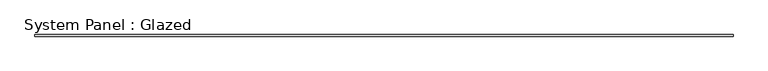
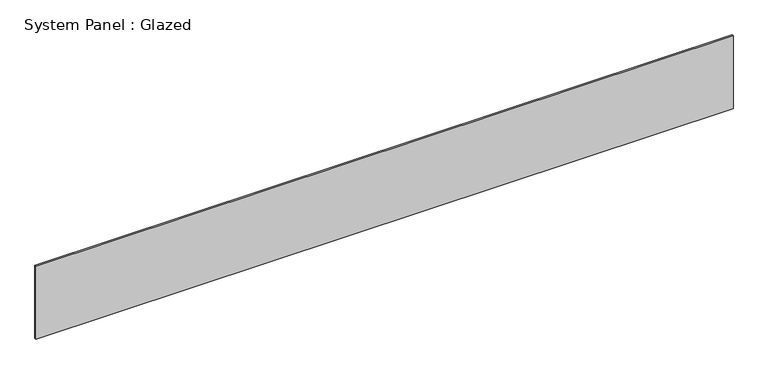
"""IFC4 building model written with IfcOpenShell, lengths in millimetres: plate geometry, System Panel : Glazed."""

from ifc_helpers import new_model, si_unit, origin, origin_with_axes, place, context, project, spatial, polyline, outline, extrude, source, transform, mapped, element, save


def system_panel_glazed_b96adab1(model_context):
    return source(origin(), model_context, "Body", "SweptSolid", [
        extrude(outline(polyline([(5520.9926253, 19.05), (-5520.9926253, 19.05), (-5520.9926253, 44.45), (5520.9926253, 44.45), (5520.9926253, 19.05)])), origin_with_axes(), (0.0, 0.0, 1.0), 1219.2),
    ])


if __name__ == "__main__":
    model = new_model("IFC4")
    model_context = context("Model", 3, world=origin())
    ifc_project = project(units=[si_unit("LENGTHUNIT", "METRE", prefix="MILLI")], contexts=[model_context])
    site = spatial("IfcSite", under=ifc_project)
    building = spatial("IfcBuilding", under=site)
    placement = place(None, origin())
    system_panel_glazed_shape = system_panel_glazed_b96adab1(model_context)
    element("IfcPlate", 1, ObjectType="System Panel : Glazed", at=placement, inside=building, context=model_context, shape_type="MappedRepresentation", body=[
        mapped(system_panel_glazed_shape, transform((0.0, 0.0, 0.0), x_axis=(1.0, 0.0, 0.0), y_axis=(0.0, 1.0, 0.0), z_axis=(0.0, 0.0, 1.0))),
    ])
    save(model, "model.ifc")

# Revit data of these elements
# Type "System Panel : Glazed"
#   Construction Type Id = "GSP4R"
#   Analytic Construction = "1/8 in Pilkington single glazing"
#   Visual Light Transmittance = 0.9
#   Solar Heat Gain Coefficient = 0.86
#   Heat Transfer Coefficient (U) = 1.18115 BTU/(h·ft²·°F)
# Element 1 (IfcPlate, "System Panel : Glazed")
#   Materials on its faces: "Glass"
# Materials
#   "Glass": class "Glass", colour RGB 0 128 192, transparency 0.75, Description = "Soda Lime Glass", Cost = 0
